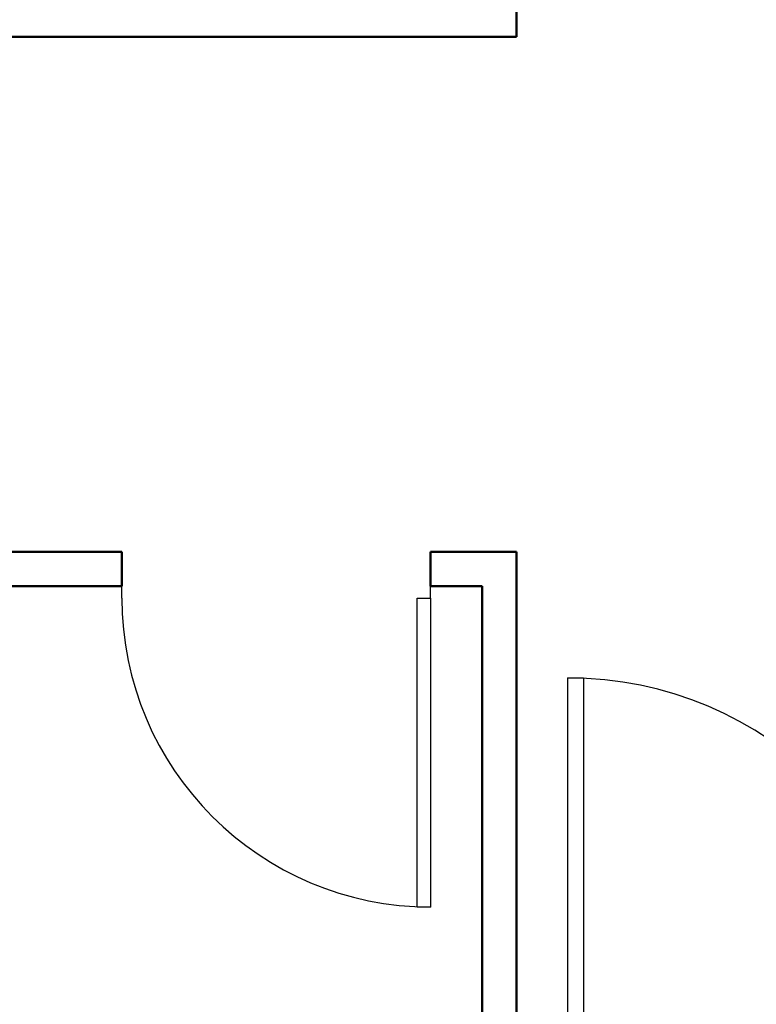
# Model space of a CAD drawing. Units: inches. Extents: x -466983 to 1020, y 324 to 318697.
# Tile 6 of 97: x 555 to 641, y 514 to 629. Entities that reach past the tile are written whole.
import ezdxf

# ---------------------------------------------------------------- set-up
doc = ezdxf.new("R2010")
doc.units = ezdxf.units.IN
doc.header["$MEASUREMENT"] = 0
for name, color, linetype, lineweight in [('A-DOOR', 3, 'Continuous', 25), ('A-FLOR-PATT', 252, 'Continuous', 13), ('A-FURN', 8, 'Continuous', 18), ('A-WALL', 7, 'Continuous', 50)]:
    doc.layers.add(name, color=color, linetype=linetype, lineweight=lineweight)

# ---------------------------------------------------------------- blocks, each defined once
blk = doc.blocks.new('A$C05F852CF')
for p, q in [((0.0306, 3.0783), (0.4692, 3.0783)), ((0.4692, 3.0783), (2.0768, 3.0783)), ((0.52, 3.0783), (0.52, 1.0783)), ((2.02, 3.0783), (2.02, 1.0783)), ((2.0768, 3.0783), (2.5066, 3.0783)), ((0, 3.0548), (0, 2.6659)), ((0.5, 3.0423), (0.5, 2.6496)), ((2.04, 3.05), (2.04, 2.6642)), ((0.52, 3.0283), (2.02, 3.0283)), ((2.54, 2.6547), (2.54, 3.0393)), ((0.2418, 2.9702), (0.2418, 3.0002)), ((0.5609, 3.0045), (0.5953, 2.9829)), ((0.5609, 3.0045), (0.6121, 2.9725)), ((1.2427, 2.9995), (1.1927, 2.9682)), ((2.2982, 2.9702), (2.2982, 3.0002)), ((0.6121, 2.9725), (0.6546, 2.9682)), ((1.1927, 2.9682), (1.1672, 2.9661)), ((0.1349, 2.8634), (0.1049, 2.8634)), ((0.3487, 2.8634), (0.3787, 2.8634)), ((2.1913, 2.8634), (2.1613, 2.8634)), ((2.4051, 2.8634), (2.4351, 2.8634)), ((0.2418, 2.7265), (0.2418, 2.7565)), ((2.2982, 2.7265), (2.2982, 2.7565)), ((0.5711, 2.6712), (0.6015, 2.7135)), ((0.6015, 2.7135), (0.6164, 2.7178)), ((1.1864, 2.7072), (1.1588, 2.7242)), ((1.2397, 2.6852), (1.1864, 2.7072)), ((1.0379, 2.6608), (0.52, 2.2697)), ((2.02, 2.6608), (1.0379, 2.6608)), ((1.7737, 2.6608), (1.7737, 1.0783)), ((1.7937, 2.6608), (1.7937, 1.0783)), ((1.8137, 2.6608), (1.8137, 1.0783)), ((1.8337, 2.6608), (1.8337, 1.0783)), ((0.0322, 2.6283), (0.4826, 2.6283)), ((2.0707, 2.6283), (2.5056, 2.6283)), ((0.52, 1.4597), (2.02, 1.4597)), ((0.52, 1.4397), (2.02, 1.4397)), ((0.52, 1.4197), (2.02, 1.4197)), ((0.52, 1.3997), (2.02, 1.3997)), ((0.52, 1.0783), (2.02, 1.0783)), ((0.726, 0.4346), (0.7377, 0.4444))]:
    blk.add_line(p, q)
for points in [[(1.3405, 2.9829), (1.306, 3.0045), (1.3573, 2.9725), (1.3998, 2.9682)], [(1.9879, 2.9995), (1.9379, 2.9682), (1.9124, 2.9661)], [(1.3162, 2.6712), (1.3467, 2.7135), (1.3616, 2.7178)], [(1.9848, 2.6852), (1.9315, 2.7072), (1.9039, 2.7242)]]:
    blk.add_lwpolyline(points)
for points in [[(1.0353, 2.1379, -0.173032), (1.022, 2.6388), (0.536, 2.2719, 0.053888)], [(1.7081, 1.7759, 0.101392), (1.7282, 1.7501, -0.223768), (1.7345, 1.736, -0.25558), (1.7315, 1.7308, -0.081563), (1.7151, 1.724, -0.071805), (1.6967, 1.7225, 0.069985), (1.6778, 1.7209, 0.03546), (1.6148, 1.7021, 0.029432), (1.5425, 1.6697, 0.001554), (1.5078, 1.6515, -0.00152), (1.4724, 1.6329, -0.004735), (1.4356, 1.6142, 0.00382), (1.3901, 1.5911, 0.296001), (1.3692, 1.5546, -0.649774), (1.3468, 1.5431, -0.02319), (1.3416, 1.5477, 0.0288), (1.3374, 1.5514, 0.005727), (1.3298, 1.557, -0.004358), (1.3198, 1.5645, -0.027528), (1.3001, 1.5812, -0.046214), (1.29, 1.5928, -0.194121), (1.2856, 1.6105, 0.133719), (1.2823, 1.6363, 0.011505), (1.2622, 1.682, 0.008882), (1.2338, 1.7401, 0.012426), (1.1937, 1.8139, -0.033612), (1.1801, 1.8418), (1.1552, 1.9026), (1.1361, 1.9495, 0.224341), (1.1204, 1.9638, -0.722772), (1.1202, 1.9734, -0.103513), (1.1242, 1.9739, 0.053465), (1.132, 1.9742, 0.030109), (1.1569, 1.9792, -0.031436), (1.1808, 1.984, -0.05324), (1.1971, 1.9844, 0.05518), (1.2128, 1.9849, 0.056271), (1.2402, 1.992, 0.0108), (1.3759, 2.0475, 0.00456), (1.4675, 2.0883, 0.01125), (1.5041, 2.106, 0.069394), (1.5235, 2.1196, -0.079756), (1.5405, 2.1311, -0.106399), (1.5562, 2.1345, -0.328642), (1.5608, 2.1312, -0.299547), (1.5587, 2.124, 0.189917), (1.5536, 2.1141, 0.033518), (1.5531, 2.1029, 0.075627), (1.554, 2.0981, 0.053489), (1.5579, 2.0898, 0.017838), (1.5727, 2.0672, 0.038394), (1.5932, 2.0425, -0.059529), (1.6058, 2.026, -0.035943), (1.6193, 1.9987, -0.011245), (1.6541, 1.9079, -0.006203), (1.6684, 1.8661, 0.010783), (1.6769, 1.8422, 0.019485), (1.6828, 1.8283, 0.005062)], [(1.6953, 1.7695, 0.098587), (1.7181, 1.7399, -0.040378), (1.7118, 1.7379, -0.071805), (1.6975, 1.7367, 0.069985), (1.6747, 1.7349, 0.03546), (1.6097, 1.7154, 0.029432), (1.5359, 1.6824, 0.001554), (1.5012, 1.6641, -0.00152), (1.4658, 1.6456, -0.004735), (1.4293, 1.627, 0.00382), (1.3835, 1.6038, 0.289814), (1.3549, 1.555, -0.018279), (1.3515, 1.5579, 0.0288), (1.3461, 1.5627, 0.005727), (1.3382, 1.5686, -0.004358), (1.3285, 1.5758, -0.027528), (1.31, 1.5916, -0.046214), (1.3016, 1.6012, -0.194121), (1.2997, 1.6085, 0.133719), (1.2955, 1.6417, 0.011505), (1.2752, 1.6881, 0.008882), (1.2465, 1.7466, 0.012426), (1.2061, 1.821, -0.033612), (1.1933, 1.8472), (1.1684, 1.908), (1.1493, 1.9549, 0.051417), (1.1455, 1.962, 0.017208), (1.1606, 1.9654, -0.031436), (1.1827, 1.9698, -0.05324), (1.196, 1.9702, 0.05518), (1.2149, 1.9708, 0.056271), (1.2453, 1.9787, 0.0108), (1.3816, 2.0344, 0.00456), (1.4734, 2.0753, 0.01125), (1.5106, 2.0933, 0.069394), (1.5332, 2.1091, -0.038161), (1.5392, 2.114, 0.029361), (1.5389, 2.1025, 0.075627), (1.5405, 2.0934, 0.053489), (1.5457, 2.0824, 0.017838), (1.5611, 2.0589, 0.038394), (1.583, 2.0326, -0.059529), (1.5935, 2.0187, -0.035943), (1.6061, 1.9933, -0.011245), (1.6406, 1.9031, -0.006203), (1.6549, 1.8617, 0.010783), (1.6635, 1.8371, 0.019485), (1.6699, 1.8222, 0.005062)]]:
    blk.add_lwpolyline(points, format="xyb", close=True)
for points in [[(1.27, 1.665, 0.025626), (1.2575, 1.662, 0.0108), (1.1179, 1.617, 0.00456), (1.0234, 1.5834, 0.01125), (0.9856, 1.5685, 0.069394), (0.9653, 1.5565, -0.079756), (0.9474, 1.5464, -0.106399), (0.9315, 1.5441, -0.328642), (0.9272, 1.5478, -0.299547), (0.9298, 1.5548, 0.189917), (0.9357, 1.5643, 0.033518), (0.9369, 1.5754, 0.075627), (0.9364, 1.5803, 0.053489), (0.9332, 1.5888, 0.017838), (0.9202, 1.6125, 0.038394), (0.9016, 1.6387, -0.059529), (0.8903, 1.6561, -0.035943), (0.8789, 1.6844, -0.011245), (0.8512, 1.7776, -0.006203), (0.8402, 1.8203, 0.010783), (0.8336, 1.8448, 0.019485), (0.8287, 1.8592, 0.005062), (0.8076, 1.9133, 0.101392), (0.7895, 1.9406, -0.223768), (0.7843, 1.9551, -0.25558), (0.7876, 1.9601, -0.081563), (0.8046, 1.9656, -0.071805), (0.823, 1.9657, 0.069985), (0.842, 1.9658, 0.03546), (0.9062, 1.9798, 0.029432), (0.9807, 2.0065, 0.001554), (1.0167, 2.022, -0.00152), (1.0535, 2.0378, -0.004735), (1.0916, 2.0536, 0.00382), (1.1388, 2.0731, 0.296001), (1.1624, 2.108, -0.649774), (1.1856, 2.1178, -0.02319), (1.1904, 2.1128, 0.0288), (1.1944, 2.1088, 0.005727), (1.2015, 2.1025, -0.004358), (1.2108, 2.0944, -0.027528), (1.2292, 2.0762, -0.046214), (1.2384, 2.0638, -0.194121), (1.2414, 2.0458, 0.133719), (1.2427, 2.0199, 0.005779), (1.2507, 1.9961)], [(1.2674, 1.6787, 0.025626), (1.2535, 1.6753, 0.0108), (1.1134, 1.6301, 0.00456), (1.0187, 1.5964, 0.01125), (0.9802, 1.5813, 0.069394), (0.9566, 1.5673, -0.042175), (0.9495, 1.5626, 0.031457), (0.9508, 1.5747, 0.075627), (0.9499, 1.5838, 0.053489), (0.9456, 1.595, 0.017838), (0.9321, 1.6196, 0.038394), (0.9123, 1.6476, -0.059529), (0.9028, 1.6622, -0.035943), (0.8922, 1.6886, -0.011245), (0.8646, 1.7812, -0.006203), (0.8536, 1.8236, 0.010783), (0.8469, 1.8487, 0.019485), (0.8417, 1.8641, 0.005062), (0.8204, 1.9185, 0.100237), (0.7996, 1.9501, -0.044209), (0.8066, 1.9519, -0.071805), (0.8211, 1.952, 0.069985), (0.8439, 1.9521, 0.03546), (0.9101, 1.9665, 0.029432), (0.9862, 1.9937, 0.001554), (1.0222, 2.0093, -0.00152), (1.0589, 2.025, -0.004735), (1.0968, 2.0408, 0.00382), (1.1442, 2.0604, 0.294287), (1.1763, 2.1074, -0.02184), (1.18, 2.1036, 0.0288), (1.1851, 2.0984, 0.005727), (1.1924, 2.092, -0.004358), (1.2016, 2.084, -0.027528), (1.2189, 2.0669, -0.046214), (1.2266, 2.0566, -0.194121), (1.2279, 2.0488, 0.133719), (1.2295, 2.0156, 0.005779), (1.2376, 1.9915, 0.005779)]]:
    blk.add_lwpolyline(points, format="xyb")
for centre, radius in [((0.2418, 2.8634), 0.1369), ((2.2982, 2.8634), 0.1369), ((0.2418, 2.8634), 0.1069), ((2.2982, 2.8634), 0.1069)]:
    blk.add_circle(centre, radius)
for centre, radius, start, end in [((1.7308, 2.407), 0.7379, 159.8846, 202.2194), ((1.4058, 4.5145), 2.4132, 248.4641, 261.4655)]:
    blk.add_arc(centre, radius, start, end)
for points in [[(0, 3.0548), (0, 3.0677), (0.0177, 3.0783), (0.0306, 3.0783)], [(0.5, 3.0423), (0.5, 3.0581), (0.485, 3.0783), (0.4692, 3.0783)], [(2.04, 3.05), (2.04, 3.0655), (2.0613, 3.0783), (2.0768, 3.0783)], [(2.5066, 3.0783), (2.5237, 3.0783), (2.54, 3.0564), (2.54, 3.0393)], [(0.0322, 2.6283), (0.0157, 2.6283), (0, 2.6494), (0, 2.6659)], [(0.5, 2.6496), (0.5, 2.6405), (0.4918, 2.6283), (0.4826, 2.6283)], [(2.04, 2.6642), (2.04, 2.6485), (2.055, 2.6283), (2.0707, 2.6283)], [(2.5056, 2.6283), (2.5201, 2.6283), (2.54, 2.6403), (2.54, 2.6547)]]:
    blk.add_open_spline(points, degree=3)
for points, knots in [([(0.5609, 3.0045), (0.565, 2.9818), (0.5836, 2.9366), (0.5776, 2.889), (0.5689, 2.8351), (0.5832, 2.7709), (0.5808, 2.7088), (0.5744, 2.6927), (0.5693, 2.6651), (0.5803, 2.6793), (0.5989, 2.6876), (0.7172, 2.6598), (0.8681, 2.7029), (1.0484, 2.6781), (1.0324, 2.6731), (1.1431, 2.7116), (1.202, 2.6757), (1.2459, 2.6867), (1.2222, 2.695), (1.2359, 2.7251), (1.2468, 2.781), (1.2288, 2.8492), (1.2515, 2.925), (1.2279, 2.9609), (1.2471, 3.0058), (1.2098, 2.9902), (1.1177, 3.0095), (0.956, 3.0159), (0.9532, 2.9758), (0.7999, 3.021), (0.7569, 3.0151), (0.5986, 2.9869), (0.561, 3.0049)], [16.816032, 16.816032, 16.816032, 16.816032, 79.038845, 88.513895, 147.565266, 227.196862, 259.685448, 283.955301, 296.511304, 302.432558, 320.230942, 354.322559, 575.279549, 734.72356, 845.740421, 943.033103, 1029.533967, 1032.845074, 1043.313584, 1065.311534, 1104.921835, 1208.53002, 1248.510714, 1303.102727, 1321.01326, 1329.647833, 1389.371624, 1571.817644, 1750.274161, 1823.189073, 1967.937033, 2020.912329, 2020.912329, 2020.912329, 2020.912329]), ([(1.306, 3.0045), (1.3102, 2.9818), (1.3287, 2.9366), (1.3228, 2.889), (1.314, 2.8351), (1.3284, 2.7709), (1.3259, 2.7088), (1.3196, 2.6927), (1.3144, 2.6651), (1.3254, 2.6793), (1.3441, 2.6876), (1.4624, 2.6598), (1.6132, 2.7029), (1.6436, 2.6781), (1.7775, 2.6731), (1.8882, 2.7116), (1.9472, 2.6757), (1.9911, 2.6867), (1.9673, 2.695), (1.981, 2.7251), (1.992, 2.781), (1.974, 2.8492), (1.9967, 2.925), (1.9731, 2.9609), (1.9922, 3.0058), (1.9549, 2.9902), (1.8628, 3.0095), (1.7011, 3.0159), (1.5483, 2.9758), (1.5451, 3.021), (1.5021, 3.0151), (1.3437, 2.9869), (1.3062, 3.0049)], [16.816032, 16.816032, 16.816032, 16.816032, 79.038845, 88.513895, 147.565266, 227.196862, 259.685448, 283.955301, 296.511304, 302.432558, 320.230942, 354.322559, 575.279549, 734.72356, 845.740421, 943.033103, 1029.533967, 1032.845074, 1043.313584, 1065.311534, 1104.921835, 1208.53002, 1248.510714, 1303.102727, 1321.01326, 1329.647833, 1389.371624, 1571.817644, 1750.274161, 1823.189073, 1967.937033, 2020.912329, 2020.912329, 2020.912329, 2020.912329]), ([(1.186, 2.943), (1.1557, 2.9456), (1.1387, 2.9502), (1.0976, 2.9551), (1.0776, 2.9567), (1.0342, 2.9582), (1.0123, 2.957), (0.991, 2.9533), (0.9902, 2.9517), (0.962, 2.9403), (0.9371, 2.935), (0.8851, 2.9413), (0.8522, 2.9513), (0.8033, 2.9629), (0.7938, 2.964), (0.755, 2.9608), (0.7319, 2.9572), (0.6794, 2.9481), (0.658, 2.9434), (0.631, 2.9418)], [1364.380335, 1364.380335, 1364.380335, 1364.380335, 1423.60231, 1423.60231, 1482.824284, 1482.824284, 1566.205036, 1566.205036, 1649.585789, 1649.585789, 1732.966542, 1732.966542, 1816.347295, 1816.347295, 1899.728048, 1899.728048, 1960.499853, 1960.499853, 1990.525565, 1990.525565, 1990.525565, 1990.525565]), ([(1.5104, 2.9621), (1.4964, 2.9606), (1.4732, 2.9568), (1.4226, 2.948), (1.4017, 2.9435), (1.3759, 2.942)], [1904.3965, 1904.3965, 1904.3965, 1904.3965, 1961.927876, 1961.927876, 1990.619445, 1990.619445, 1990.619445, 1990.619445]), ([(1.9314, 2.9432), (1.8997, 2.9459), (1.8822, 2.9507), (1.8387, 2.9557), (1.8168, 2.9572), (1.7515, 2.9587), (1.7088, 2.9551), (1.6403, 2.9447), (1.6154, 2.9402), (1.5795, 2.937), (1.5675, 2.9361), (1.5394, 2.9412), (1.5201, 2.9507), (1.5104, 2.9621)], [1364.265661, 1364.265661, 1364.265661, 1364.265661, 1426.240795, 1426.240795, 1488.215928, 1488.215928, 1612.166195, 1612.166195, 1689.92864, 1689.92864, 1733.064362, 1733.064362, 1768.978829, 1768.978829, 1768.978829, 1768.978829]), ([(0.631, 2.9418), (0.6332, 2.9288), (0.633, 2.9104), (0.6308, 2.893), (0.6298, 2.8865), (0.628, 2.8726), (0.6273, 2.866), (0.6257, 2.8474), (0.6257, 2.8375), (0.629, 2.8013), (0.6345, 2.7696), (0.6337, 2.7333)], [67.285362, 67.285362, 67.285362, 67.285362, 87.399558, 87.399558, 107.513754, 107.513754, 127.62795, 127.62795, 167.856341, 167.856341, 238.127268, 238.127268, 238.127268, 238.127268]), ([(1.1845, 2.7412), (1.189, 2.7552), (1.1894, 2.765), (1.1874, 2.7998), (1.1843, 2.8219), (1.1844, 2.8664), (1.1882, 2.8901), (1.192, 2.9105), (1.1922, 2.9144), (1.1921, 2.9158), (1.1908, 2.9212), (1.1875, 2.9351), (1.1867, 2.9388), (1.186, 2.943)], [1072.516901, 1072.516901, 1072.516901, 1072.516901, 1129.100964, 1129.100964, 1185.685027, 1185.685027, 1226.035089, 1226.035089, 1249.281274, 1249.281274, 1272.52746, 1272.52746, 1279.689275, 1279.689275, 1279.689275, 1279.689275]), ([(1.3759, 2.942), (1.3781, 2.929), (1.378, 2.9106), (1.3757, 2.893), (1.3748, 2.8866), (1.373, 2.8727), (1.3722, 2.8661), (1.3706, 2.8475), (1.3707, 2.8375), (1.3739, 2.8012), (1.3795, 2.7694), (1.3787, 2.7331)], [67.156228, 67.156228, 67.156228, 67.156228, 87.297212, 87.297212, 107.438196, 107.438196, 127.57918, 127.57918, 167.861148, 167.861148, 238.25357, 238.25357, 238.25357, 238.25357]), ([(1.9299, 2.7409), (1.9344, 2.755), (1.9348, 2.7648), (1.9328, 2.7996), (1.9297, 2.8217), (1.9298, 2.8662), (1.9336, 2.8899), (1.9374, 2.9105), (1.9376, 2.9144), (1.9375, 2.9159), (1.9362, 2.9214), (1.9329, 2.9353), (1.9321, 2.939), (1.9314, 2.9432)], [1072.238498, 1072.238498, 1072.238498, 1072.238498, 1128.864869, 1128.864869, 1185.491239, 1185.491239, 1225.989553, 1225.989553, 1249.326401, 1249.326401, 1272.66325, 1272.66325, 1279.788508, 1279.788508, 1279.788508, 1279.788508]), ([(0.6337, 2.7333), (0.6515, 2.7301), (0.6627, 2.7284), (0.6898, 2.7263), (0.7032, 2.726), (0.7436, 2.727), (0.7707, 2.73), (0.8409, 2.7383), (0.8881, 2.7432), (0.9755, 2.7406), (1.0125, 2.7357), (1.0356, 2.7309), (1.0369, 2.7307), (1.0381, 2.7304)], [345.4047, 345.4047, 345.4047, 345.4047, 383.386056, 383.386056, 421.367413, 421.367413, 497.330126, 497.330126, 611.561469, 611.561469, 725.792813, 725.792813, 732.434768, 732.434768, 732.434768, 732.434768]), ([(1.0381, 2.7304), (1.0497, 2.7345), (1.0742, 2.7435), (1.1251, 2.7504), (1.1528, 2.749), (1.1769, 2.7432), (1.1809, 2.7421), (1.1845, 2.7412)], [843.64503, 843.64503, 843.64503, 843.64503, 911.27572, 911.27572, 959.088062, 959.088062, 969.47998, 969.47998, 969.47998, 969.47998]), ([(1.3787, 2.7331), (1.3984, 2.7296), (1.4106, 2.7278), (1.4401, 2.7258), (1.4545, 2.7258), (1.4962, 2.7276), (1.5219, 2.7313), (1.5767, 2.7399), (1.6067, 2.7436), (1.6527, 2.7371), (1.662, 2.7326), (1.7084, 2.7282), (1.7364, 2.7276), (1.7849, 2.734), (1.8076, 2.7406), (1.8563, 2.7489), (1.8812, 2.7508), (1.914, 2.7451), (1.9226, 2.7428), (1.9299, 2.7409)], [345.267918, 345.267918, 345.267918, 345.267918, 387.167414, 387.167414, 429.06691, 429.06691, 512.865903, 512.865903, 629.317545, 629.317545, 745.769188, 745.769188, 834.622813, 834.622813, 901.414409, 901.414409, 948.921878, 948.921878, 969.679511, 969.679511, 969.679511, 969.679511])]:
    blk.add_open_spline(points, degree=3, knots=knots)
for p in [(0.2366, 2.8475), (2.3034, 2.8475), (0.2309, 2.8244), (2.02, 1.0783), (2.02, 1.0783)]:
    blk.add_point(p)
blk = doc.blocks.new('*U37')
for p, q in [((-40, 0), (-40, 6)), ((0, 0), (0, 6))]:
    blk.add_line(p, q)
blk.add_lwpolyline([(0, 0), (0, -40), (-1.75, -40), (-1.75, 0)], close=True)
blk.add_arc((0, 0), 40, 180, 270)
blk = doc.blocks.new('*U41')
for p, q in [((0, 0), (0, -6)), ((40, 0), (40, -6))]:
    blk.add_line(p, q)
blk.add_lwpolyline([(0, 0), (0, 40), (1.75, 40), (1.75, 0)], close=True)
blk.add_arc((0, 0), 40, 0, 90)

msp = doc.modelspace()

# ---------------------------------------------------------------- hatches: boundary and pattern name
at = {"layer": 'A-FLOR-PATT', "transparency": 33554572}
h = msp.add_hatch(dxfattribs=at)
h.set_pattern_fill('ANSI37', color=256, scale=30)
h.set_pattern_definition([(45, (-1212.4137, -290.035), (-2.6516504, 2.6516504), []), (135, (-1212.4137, -290.035), (-2.6516504, -2.6516504), [])])
h.paths.add_polyline_path([(901.81, 1075.94), (900.61, 1075.94), (900.61, 1065.39), (899.39, 1065.39), (898.09, 1065.39), (892.84, 1058.71, -0.258377), (892.19, 1058.35), (879.98, 1058.35, -0.20177), (879.44, 1058.58), (874.08, 1065.39), (872.78, 1065.39), (871.56, 1065.39), (871.56, 1075.94), (813.81, 1075.94), (813.81, 1044.79), (832.39, 1044.79, -0.394795), (848.66, 1028.54), (848.66, 1009.94), (901.81, 1009.94), (901.81, 1015.94), (901.31, 1015.94), (871.31, 1015.94), (871.31, 1017.25), (871.33, 1017.25, -0.401453), (901.31, 1045.94), (901.81, 1045.94)])
edge = h.paths.add_edge_path(flags=16)
edge.add_line((847.77, 1068.95), (847.77, 1073.71))
edge.add_arc((849.23, 1073.71), 1.45, 90, 180, ccw=False)
edge.add_line((849.23, 1075.16), (864.49, 1075.16))
edge.add_arc((864.49, 1073.71), 1.45, 0, 90, ccw=False)
edge.add_line((865.95, 1073.71), (865.95, 1069))
edge.add_arc((832.64, 1068.98), 33.3, -20.6123, 0.0472, ccw=False)
edge.add_ellipse((856.86, 1058.48), major_axis=(0, 10.21), ratio=0.685919, start_angle=100.0088, end_angle=259.9912, ccw=False)
edge.add_arc((881.07, 1068.98), 33.3, 180.0472, 200.6123, ccw=False)
h.paths.add_polyline_path([(853.15, 1066.48), (853.15, 1066.45), (853.15, 1066.45, 0.433107), (852.92, 1066.68), (852.92, 1066.45), (853.15, 1066.45), (853.15, 1066.48), (853.09, 1066.61, 0.697939), (852.7, 1066.45), (852.7, 1066.45), (852.7, 1066.48), (852.92, 1067), (852.92, 1066.68, -0.396254)], flags=0)
h.paths.add_polyline_path([(861.02, 1066.48), (861.02, 1066.45), (861.02, 1066.45, 0.416404), (860.8, 1066.68), (860.8, 1066.45), (861.02, 1066.45), (861.02, 1066.48), (860.97, 1066.61, 0.713344), (860.57, 1066.45), (860.57, 1066.45), (860.57, 1066.48), (860.8, 1067), (860.8, 1066.68, -0.379973)], flags=0)
edge = h.paths.add_edge_path(flags=0)
edge.add_spline(control_points=[(861.13, 1065.79), (861.47, 1065.25), (861.61, 1065.02), (861.98, 1064.37), (862.19, 1063.94), (862.56, 1063.04), (862.72, 1062.56), (862.99, 1061.58), (863.09, 1061.07), (863.25, 1060.03), (863.29, 1059.5), (863.33, 1058.44), (863.32, 1057.91), (863.24, 1056.85), (863.17, 1056.33), (862.97, 1055.31), (862.84, 1054.81), (862.54, 1053.85), (862.36, 1053.39), (861.95, 1052.52), (861.73, 1052.12), (861.23, 1051.36), (860.97, 1051.02), (860.4, 1050.39), (860.11, 1050.12), (859.49, 1049.65), (859.18, 1049.45), (858.53, 1049.13), (858.2, 1049.01), (857.53, 1048.85), (857.2, 1048.81), (856.52, 1048.81), (856.19, 1048.85), (855.52, 1049.01), (855.19, 1049.13), (854.54, 1049.45), (854.23, 1049.64), (853.61, 1050.12), (853.32, 1050.39), (852.75, 1051.01), (852.49, 1051.36), (852, 1052.11), (851.77, 1052.52), (851.36, 1053.39), (851.18, 1053.85), (850.88, 1054.81), (850.75, 1055.31), (850.55, 1056.33), (850.48, 1056.85), (850.4, 1057.9), (850.39, 1058.44), (850.43, 1059.5), (850.47, 1060.03), (850.63, 1061.07), (850.73, 1061.58), (851, 1062.56), (851.16, 1063.04), (851.53, 1063.94), (851.73, 1064.37), (852.11, 1065.02), (852.25, 1065.25), (852.61, 1065.73)], knot_values=[3.915332, 3.915332, 3.915332, 3.915332, 4.013468, 4.013468, 4.175532, 4.175532, 4.337596, 4.337596, 4.49966, 4.49966, 4.661724, 4.661724, 4.823788, 4.823788, 4.985852, 4.985852, 5.147916, 5.147916, 5.30998, 5.30998, 5.472044, 5.472044, 5.634109, 5.634109, 5.796173, 5.796173, 5.958237, 5.958237, 6.120301, 6.120301, 6.282365, 6.282365, 6.444429, 6.444429, 6.606493, 6.606493, 6.768557, 6.768557, 6.930621, 6.930621, 7.092685, 7.092685, 7.254749, 7.254749, 7.416813, 7.416813, 7.578878, 7.578878, 7.740942, 7.740942, 7.903006, 7.903006, 8.06507, 8.06507, 8.227134, 8.227134, 8.389198, 8.389198, 8.551262, 8.551262, 8.65037, 8.65037, 8.65037, 8.65037], degree=3, periodic=0)
edge.add_line((852.64, 1065.79), (861.13, 1065.79))
edge = h.paths.add_edge_path(flags=0)
edge.add_ellipse((856.85, 1057.74), major_axis=(0, 7.79), ratio=0.687861, start_angle=0, end_angle=360)
h.paths.add_polyline_path([(848.86, 1069.39), (848.86, 1073.96, -0.414214), (849.95, 1075.05), (863.77, 1075.05, -0.414214), (864.86, 1073.96), (864.86, 1069.39, -0.388936), (864.52, 1069.03, -0.043561), (849.2, 1069.03, -0.388936)], flags=0)
h.paths.add_polyline_path([(853.1, 1068.11, -1), (852.68, 1068.11, -1)], flags=0)
edge = h.paths.add_edge_path(flags=0)
edge.add_ellipse((856.86, 1057.34), major_axis=(0, 2.21), ratio=0.657164, start_angle=0, end_angle=360)
h.paths.add_polyline_path([(861.04, 1068.11, -1), (860.62, 1068.11, -1)], flags=0)
edge = h.paths.add_edge_path()
edge.add_line((573.95, 1057.34), (573.95, 1075.94))
edge.add_line((573.95, 1075.94), (558.73, 1075.94))
edge.add_line((558.73, 1075.94), (558.73, 1065.39))
edge.add_line((558.73, 1065.39), (557.51, 1065.39))
edge.add_line((557.51, 1065.39), (556.21, 1065.39))
edge.add_line((556.21, 1065.39), (550.95, 1058.71))
edge.add_arc((550.3, 1059.12), 0.765, 270, 327.9483, ccw=False)
edge.add_line((550.3, 1058.35), (538.1, 1058.35))
edge.add_arc((538.1, 1059.12), 0.765, 224.3704, 270, ccw=False)
edge.add_line((537.55, 1058.58), (532.2, 1065.39))
edge.add_line((532.2, 1065.39), (530.9, 1065.39))
edge.add_line((530.9, 1065.39), (529.67, 1065.39))
edge.add_line((529.67, 1065.39), (529.67, 1075.94))
edge.add_line((529.67, 1075.94), (520.81, 1075.94))
edge.add_line((520.81, 1075.94), (520.81, 1045.94))
edge.add_line((520.81, 1045.94), (521.31, 1045.94))
edge.add_arc((521.31, 1015.94), 30, 2.5075, 90, ccw=False)
edge.add_line((551.28, 1017.25), (551.31, 1017.25))
edge.add_line((551.31, 1017.25), (551.31, 1015.94))
edge.add_line((551.31, 1015.94), (520.81, 1015.94))
edge.add_line((520.81, 1015.94), (520.81, 1009.94))
edge.add_line((520.81, 1009.94), (559.19, 1010.4))
edge.add_arc((559.19, 1011.86), 1.45, 180, 270, ccw=False)
edge.add_line((557.74, 1011.86), (557.74, 1016.56))
edge.add_arc((591.04, 1016.59), 33.3, 159.3877, 180.0472, ccw=False)
edge.add_ellipse((566.82, 1027.08), major_axis=(0, 10.21), ratio=0.685919, start_angle=280.0088, end_angle=439.9912, ccw=False)
edge.add_arc((542.61, 1016.59), 33.3, 0.0472, 20.6123, ccw=False)
edge.add_line((575.91, 1016.62), (575.91, 1011.86))
edge.add_arc((574.46, 1011.86), 1.45, -90, 0, ccw=False)
edge.add_line((574.46, 1010.4), (608.81, 1009.94))
edge.add_line((608.81, 1009.94), (608.81, 1041.09))
edge.add_line((608.81, 1041.09), (590.22, 1041.09))
edge.add_arc((590.78, 1057.91), 16.83, 181.9277, 268.1032, ccw=False)
edge = h.paths.add_edge_path()
edge.add_ellipse((494.24, 583.62), major_axis=(0, 10.21), ratio=0.685919, start_angle=280.0088, end_angle=439.9912, ccw=False)
edge.add_arc((470.03, 573.12), 33.3, 0.0472, 20.6123, ccw=False)
edge.add_line((503.33, 573.15), (503.33, 568.39))
edge.add_arc((501.88, 568.39), 1.45, -90, 0, ccw=False)
edge.add_line((501.88, 566.94), (539.81, 566.94))
edge.add_line((539.81, 566.94), (539.81, 572.94))
edge.add_line((539.81, 572.94), (539.31, 572.94))
edge.add_line((539.31, 572.94), (509.31, 572.94))
edge.add_line((509.31, 572.94), (509.31, 574.25))
edge.add_line((509.31, 574.25), (509.33, 574.25))
edge.add_arc((539.31, 572.94), 30, 90, 177.4925, ccw=False)
edge.add_line((539.31, 602.94), (539.81, 602.94))
edge.add_line((539.81, 602.94), (539.81, 626.94))
edge.add_line((539.81, 626.94), (531.77, 626.94))
edge.add_line((531.77, 626.94), (531.77, 616.39))
edge.add_line((531.77, 616.39), (530.55, 616.39))
edge.add_line((530.55, 616.39), (529.25, 616.39))
edge.add_line((529.25, 616.39), (523.71, 609.35))
edge.add_line((523.71, 609.35), (510.78, 609.35))
edge.add_line((510.78, 609.35), (505.24, 616.39))
edge.add_line((505.24, 616.39), (503.94, 616.39))
edge.add_line((503.94, 616.39), (502.72, 616.39))
edge.add_line((502.72, 616.39), (502.72, 626.94))
edge.add_line((502.72, 626.94), (481.7, 626.94))
edge.add_line((481.7, 626.94), (481.7, 611))
edge.add_arc((467.27, 611.47), 14.44, 271.9277, 358.1032, ccw=False)
edge.add_line((467.76, 597.05), (451.81, 597.05))
edge.add_line((451.81, 597.05), (451.81, 584.4))
edge.add_line((451.81, 584.4), (451.81, 566.94))
edge.add_line((451.81, 566.94), (486.61, 566.94))
edge.add_arc((486.61, 568.39), 1.45, 180, 270, ccw=False)
edge.add_line((485.16, 568.39), (485.16, 573.1))
edge.add_arc((518.46, 573.12), 33.3, 159.3877, 180.0472, ccw=False)
h.paths.add_polyline_path([(836.26, 1020.73), (879.89, 1020.73), (879.89, 1039.39), (836.26, 1039.39)], flags=25)
h.paths.add_polyline_path([(549.99, 1036.75), (593.61, 1036.75), (593.61, 1055.41), (549.99, 1055.41)], flags=24)
h.paths.add_polyline_path([(475.12, 595.6), (518.75, 595.6), (518.75, 614.25), (475.12, 614.25)], flags=24)

# ---------------------------------------------------------------- linework, layer by layer
at = {"layer": 'A-WALL'}
for p, q in [((612.81, 626.94), (612.81, 748.94)), ((612.81, 626.94), (543.81, 626.94)), ((566.81, 566.94), (543.81, 566.94)), ((566.81, 562.94), (566.81, 566.94)), ((612.81, 566.94), (602.81, 566.94)), ((602.81, 562.94), (602.81, 566.94)), ((612.81, 415.94), (612.81, 566.94)), ((566.81, 562.94), (451.81, 562.94)), ((608.81, 562.94), (602.81, 562.94)), ((608.81, 424.94), (608.81, 562.94))]:
    msp.add_line(p, q, dxfattribs=at)

# ---------------------------------------------------------------- block references
at = {"layer": 'A-DOOR'}
for name, p, xscale, yscale, zscale in [('*U37', (602.81, 561.54), 0.9, 0.9, 0.9), ('*U41', (618.81, 510.24), 1.05, 1.05, 1.05)]:
    msp.add_blockref(name, p, dxfattribs=dict(at, xscale=xscale, yscale=yscale, zscale=zscale))
at = {"layer": 'A-FURN', "xscale": 40, "yscale": 40, "zscale": 40, "rotation": 180}
msp.add_blockref('A$C05F852CF', (576.97, 548.49), dxfattribs=at)

doc.saveas('drawing.dxf')
